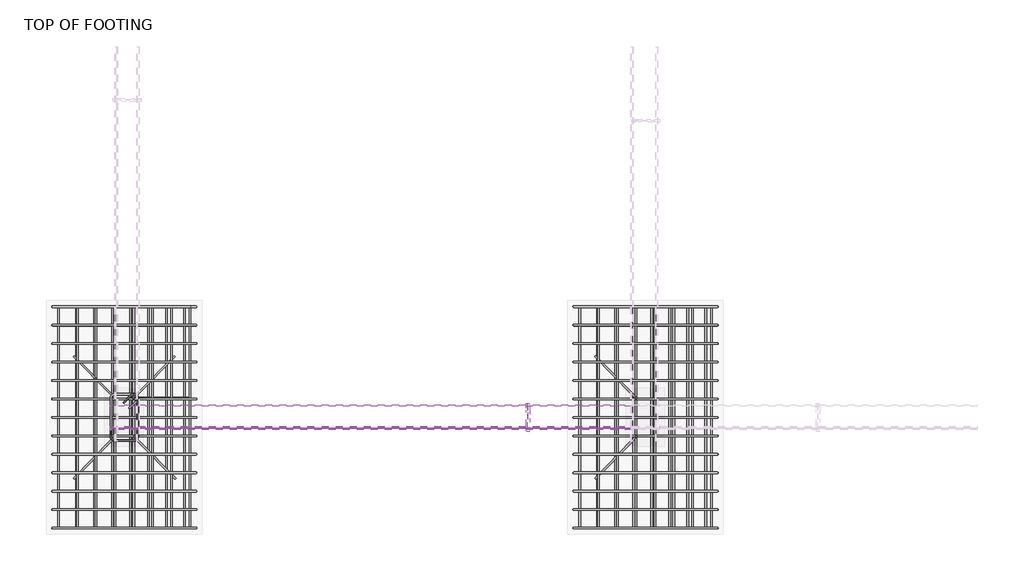
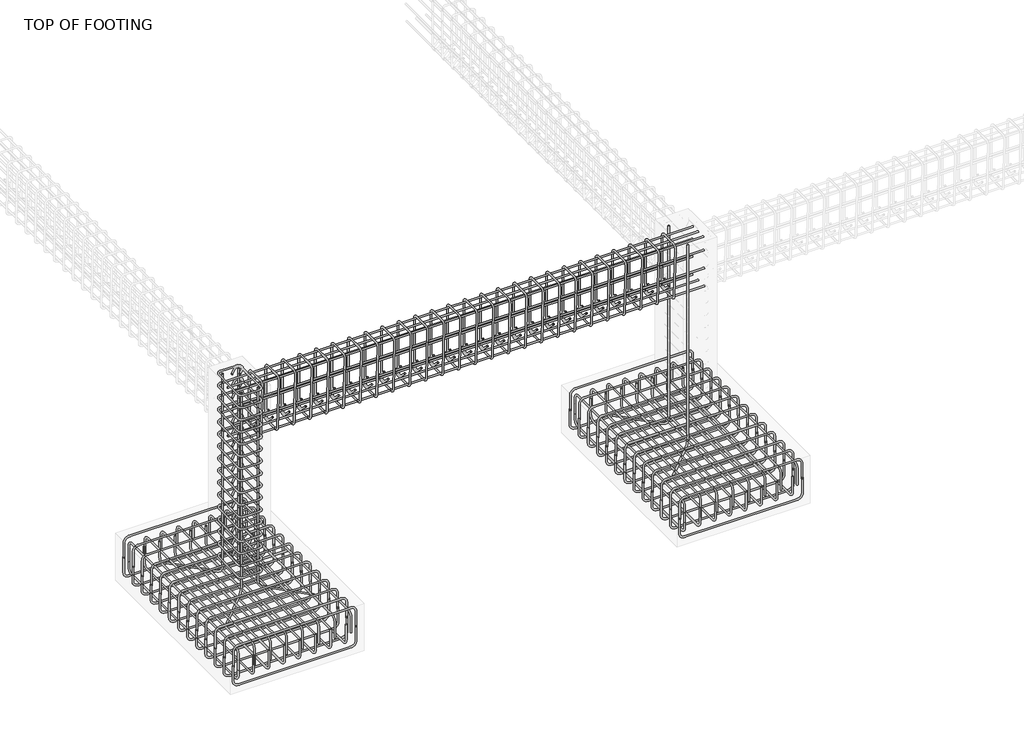
# One storey, part 2 of 21: 23 reinforcing bars.
"""IFC4 building model written with IfcOpenShell, lengths in millimetres."""

from ifc_helpers import new_model, si_unit, point, frame, origin, place, context, project, spatial, polyline, circle_curve, trimmed, segment, composite_curve, source, transform, mapped, element, save
from ifc_brep_helpers import swept_disk

model = new_model("IFC4")

# Units and contexts
model_context = context("Model", 3, world=origin())
ifc_project = project(units=[si_unit("LENGTHUNIT", "METRE", prefix="MILLI")], contexts=[model_context])

# Site, building, storey
site = spatial("IfcSite", under=ifc_project)
building = spatial("IfcBuilding", under=site)
storey = spatial("IfcBuildingStorey", under=building, Name="TOP OF FOOTING", Elevation=-1828.8)

# Reinforcing bars
placement = place(None, origin())
reinforcing_bar_shape = source(origin(), model_context, "Body", "SolidModel", [
    swept_disk(composite_curve([segment(polyline([(-13268.2584825, 443.1886958, -2045.4168622), (-13268.2584825, 443.1886958, -2192.7168622)]), True, "CONTINUOUS"), segment(trimmed(circle_curve(frame((-13314.6084825, 443.1886958, -2192.7168622), z_axis=(0.0, 1.0, 0.0), x_axis=(46.350000000000364, 0.0, 0.0)), 46.35), [point((-13268.2584825, 443.1886958, -2192.7168622))], [point((-13314.6084825, 443.1886958, -2239.0668622))], True, "CARTESIAN"), True, "CONTINUOUS"), segment(polyline([(-13314.6084825, 443.1886958, -2239.0668622), (-14329.2084825, 443.1886958, -2239.0668622)]), True, "CONTINUOUS"), segment(trimmed(circle_curve(frame((-14329.2084825, 443.1886958, -2192.7168622), z_axis=(0.0, 1.0, 0.0), x_axis=(0.0, 0.0, -46.34999999999991)), 46.35), [point((-14329.2084825, 443.1886958, -2239.0668622))], [point((-14375.5584825, 443.1886958, -2192.7168622))], True, "CARTESIAN"), True, "CONTINUOUS"), segment(polyline([(-14375.5584825, 443.1886958, -2192.7168622), (-14375.5584825, 443.1886958, -2045.4168622)]), True, "CONTINUOUS")], self_intersect=False), 6.35),
])
element("IfcReinforcingBar", 1, at=placement, inside=storey, context=model_context, shape_type="MappedRepresentation", body=[
    mapped(reinforcing_bar_shape, transform((0.0, 0.0, 0.0), x_axis=(1.0, 0.0, 0.0), y_axis=(0.0, 1.0, 0.0), z_axis=(0.0, 0.0, 1.0))),
    mapped(reinforcing_bar_shape, transform((0.0, -142.275, 0.0), x_axis=(1.0, 0.0, 0.0), y_axis=(0.0, 1.0, 0.0), z_axis=(0.0, 0.0, 1.0))),
    mapped(reinforcing_bar_shape, transform((0.0, -284.55, 0.0), x_axis=(1.0, 0.0, 0.0), y_axis=(0.0, 1.0, 0.0), z_axis=(0.0, 0.0, 1.0))),
    mapped(reinforcing_bar_shape, transform((0.0, -426.825, 0.0), x_axis=(1.0, 0.0, 0.0), y_axis=(0.0, 1.0, 0.0), z_axis=(0.0, 0.0, 1.0))),
    mapped(reinforcing_bar_shape, transform((0.0, -569.1, 0.0), x_axis=(1.0, 0.0, 0.0), y_axis=(0.0, 1.0, 0.0), z_axis=(0.0, 0.0, 1.0))),
    mapped(reinforcing_bar_shape, transform((0.0, -711.375, 0.0), x_axis=(1.0, 0.0, 0.0), y_axis=(0.0, 1.0, 0.0), z_axis=(0.0, 0.0, 1.0))),
    mapped(reinforcing_bar_shape, transform((0.0, -853.65, 0.0), x_axis=(1.0, 0.0, 0.0), y_axis=(0.0, 1.0, 0.0), z_axis=(0.0, 0.0, 1.0))),
    mapped(reinforcing_bar_shape, transform((0.0, -995.925, 0.0), x_axis=(1.0, 0.0, 0.0), y_axis=(0.0, 1.0, 0.0), z_axis=(0.0, 0.0, 1.0))),
    mapped(reinforcing_bar_shape, transform((0.0, -1138.2, 0.0), x_axis=(1.0, 0.0, 0.0), y_axis=(0.0, 1.0, 0.0), z_axis=(0.0, 0.0, 1.0))),
    mapped(reinforcing_bar_shape, transform((0.0, -1280.475, 0.0), x_axis=(1.0, 0.0, 0.0), y_axis=(0.0, 1.0, 0.0), z_axis=(0.0, 0.0, 1.0))),
    mapped(reinforcing_bar_shape, transform((0.0, -1422.75, 0.0), x_axis=(1.0, 0.0, 0.0), y_axis=(0.0, 1.0, 0.0), z_axis=(0.0, 0.0, 1.0))),
    mapped(reinforcing_bar_shape, transform((0.0, -1565.025, 0.0), x_axis=(1.0, 0.0, 0.0), y_axis=(0.0, 1.0, 0.0), z_axis=(0.0, 0.0, 1.0))),
    mapped(reinforcing_bar_shape, transform((0.0, -1707.3, 0.0), x_axis=(1.0, 0.0, 0.0), y_axis=(0.0, 1.0, 0.0), z_axis=(0.0, 0.0, 1.0))),
])
reinforcing_bar_2_shape = source(origin(), model_context, "Body", "SolidModel", [
    swept_disk(composite_curve([segment(polyline([(-14372.2274202, 443.1886958, -2057.1074344), (-14372.2274202, 443.1886958, -1909.8074344)]), True, "CONTINUOUS"), segment(trimmed(circle_curve(frame((-14325.8774202, 443.1886958, -1909.8074344), z_axis=(0.0, 1.0, 0.0), x_axis=(-46.350000000000364, 0.0, 0.0)), 46.35), [point((-14372.2274202, 443.1886958, -1909.8074344))], [point((-14325.8774202, 443.1886958, -1863.4574344))], True, "CARTESIAN"), True, "CONTINUOUS"), segment(polyline([(-14325.8774202, 443.1886958, -1863.4574344), (-13316.98705, 443.1886958, -1863.4574344)]), True, "CONTINUOUS"), segment(trimmed(circle_curve(frame((-13316.98705, 443.1886958, -1909.8074344), z_axis=(0.0, 1.0, 0.0), x_axis=(0.0, 0.0, 46.34999999999991)), 46.35), [point((-13316.98705, 443.1886958, -1863.4574344))], [point((-13270.63705, 443.1886958, -1909.8074344))], True, "CARTESIAN"), True, "CONTINUOUS"), segment(polyline([(-13270.63705, 443.1886958, -1909.8074344), (-13270.63705, 443.1886958, -2057.1074344)]), True, "CONTINUOUS")], self_intersect=False), 6.35),
])
element("IfcReinforcingBar", 2, at=placement, inside=storey, context=model_context, shape_type="MappedRepresentation", body=[
    mapped(reinforcing_bar_2_shape, transform((0.0, 0.0, 0.0), x_axis=(1.0, 0.0, 0.0), y_axis=(0.0, 1.0, 0.0), z_axis=(0.0, 0.0, 1.0))),
    mapped(reinforcing_bar_2_shape, transform((0.0, -142.275, 0.0), x_axis=(1.0, 0.0, 0.0), y_axis=(0.0, 1.0, 0.0), z_axis=(0.0, 0.0, 1.0))),
    mapped(reinforcing_bar_2_shape, transform((0.0, -284.55, 0.0), x_axis=(1.0, 0.0, 0.0), y_axis=(0.0, 1.0, 0.0), z_axis=(0.0, 0.0, 1.0))),
    mapped(reinforcing_bar_2_shape, transform((0.0, -426.825, 0.0), x_axis=(1.0, 0.0, 0.0), y_axis=(0.0, 1.0, 0.0), z_axis=(0.0, 0.0, 1.0))),
    mapped(reinforcing_bar_2_shape, transform((0.0, -569.1, 0.0), x_axis=(1.0, 0.0, 0.0), y_axis=(0.0, 1.0, 0.0), z_axis=(0.0, 0.0, 1.0))),
    mapped(reinforcing_bar_2_shape, transform((0.0, -711.375, 0.0), x_axis=(1.0, 0.0, 0.0), y_axis=(0.0, 1.0, 0.0), z_axis=(0.0, 0.0, 1.0))),
    mapped(reinforcing_bar_2_shape, transform((0.0, -853.65, 0.0), x_axis=(1.0, 0.0, 0.0), y_axis=(0.0, 1.0, 0.0), z_axis=(0.0, 0.0, 1.0))),
    mapped(reinforcing_bar_2_shape, transform((0.0, -995.925, 0.0), x_axis=(1.0, 0.0, 0.0), y_axis=(0.0, 1.0, 0.0), z_axis=(0.0, 0.0, 1.0))),
    mapped(reinforcing_bar_2_shape, transform((0.0, -1138.2, 0.0), x_axis=(1.0, 0.0, 0.0), y_axis=(0.0, 1.0, 0.0), z_axis=(0.0, 0.0, 1.0))),
    mapped(reinforcing_bar_2_shape, transform((0.0, -1280.475, 0.0), x_axis=(1.0, 0.0, 0.0), y_axis=(0.0, 1.0, 0.0), z_axis=(0.0, 0.0, 1.0))),
    mapped(reinforcing_bar_2_shape, transform((0.0, -1422.75, 0.0), x_axis=(1.0, 0.0, 0.0), y_axis=(0.0, 1.0, 0.0), z_axis=(0.0, 0.0, 1.0))),
    mapped(reinforcing_bar_2_shape, transform((0.0, -1565.025, 0.0), x_axis=(1.0, 0.0, 0.0), y_axis=(0.0, 1.0, 0.0), z_axis=(0.0, 0.0, 1.0))),
    mapped(reinforcing_bar_2_shape, transform((0.0, -1707.3, 0.0), x_axis=(1.0, 0.0, 0.0), y_axis=(0.0, 1.0, 0.0), z_axis=(0.0, 0.0, 1.0))),
])
reinforcing_bar_3_shape = source(origin(), model_context, "Body", "SolidModel", [
    swept_disk(composite_curve([segment(polyline([(-13314.2120502, 443.1886958, -2099.3509187), (-13314.2120502, 443.1886958, -1952.0509187)]), True, "CONTINUOUS"), segment(trimmed(circle_curve(frame((-13314.2120502, 396.8386958, -1952.0509187), z_axis=(1.0, 0.0, 0.0), x_axis=(0.0, 46.35000000000002, 0.0)), 46.35), [point((-13314.2120502, 443.1886958, -1952.0509187))], [point((-13314.2120502, 396.8386958, -1905.7009187))], True, "CARTESIAN"), True, "CONTINUOUS"), segment(polyline([(-13314.2120502, 396.8386958, -1905.7009187), (-13314.2120502, -1217.7613042, -1905.7009187)]), True, "CONTINUOUS"), segment(trimmed(circle_curve(frame((-13314.2120502, -1217.7613042, -1952.0509187), z_axis=(1.0, 0.0, 0.0), x_axis=(0.0, 0.0, 46.34999999999991)), 46.35), [point((-13314.2120502, -1217.7613042, -1905.7009187))], [point((-13314.2120502, -1264.1113042, -1952.0509187))], True, "CARTESIAN"), True, "CONTINUOUS"), segment(polyline([(-13314.2120502, -1264.1113042, -1952.0509187), (-13314.2120502, -1264.1113042, -2099.3509187)]), True, "CONTINUOUS")], self_intersect=False), 6.35),
])
element("IfcReinforcingBar", 3, at=placement, inside=storey, context=model_context, shape_type="MappedRepresentation", body=[
    mapped(reinforcing_bar_3_shape, transform((0.0, 0.0, 0.0), x_axis=(1.0, 0.0, 0.0), y_axis=(0.0, 1.0, 0.0), z_axis=(0.0, 0.0, 1.0))),
    mapped(reinforcing_bar_3_shape, transform((-145.0295561, 0.0, 0.0), x_axis=(1.0, 0.0, 0.0), y_axis=(0.0, 1.0, 0.0), z_axis=(0.0, 0.0, 1.0))),
    mapped(reinforcing_bar_3_shape, transform((-290.0591123, 0.0, 0.0), x_axis=(1.0, 0.0, 0.0), y_axis=(0.0, 1.0, 0.0), z_axis=(0.0, 0.0, 1.0))),
    mapped(reinforcing_bar_3_shape, transform((-435.0886684, 0.0, 0.0), x_axis=(1.0, 0.0, 0.0), y_axis=(0.0, 1.0, 0.0), z_axis=(0.0, 0.0, 1.0))),
    mapped(reinforcing_bar_3_shape, transform((-580.1182245, 0.0, 0.0), x_axis=(1.0, 0.0, 0.0), y_axis=(0.0, 1.0, 0.0), z_axis=(0.0, 0.0, 1.0))),
    mapped(reinforcing_bar_3_shape, transform((-725.1477807, 0.0, 0.0), x_axis=(1.0, 0.0, 0.0), y_axis=(0.0, 1.0, 0.0), z_axis=(0.0, 0.0, 1.0))),
    mapped(reinforcing_bar_3_shape, transform((-870.1773368, 0.0, 0.0), x_axis=(1.0, 0.0, 0.0), y_axis=(0.0, 1.0, 0.0), z_axis=(0.0, 0.0, 1.0))),
    mapped(reinforcing_bar_3_shape, transform((-1015.206893, 0.0, 0.0), x_axis=(1.0, 0.0, 0.0), y_axis=(0.0, 1.0, 0.0), z_axis=(0.0, 0.0, 1.0))),
])
reinforcing_bar_4_shape = source(origin(), model_context, "Body", "SolidModel", [
    swept_disk(composite_curve([segment(polyline([(-14329.4189432, 443.1886958, -2006.0306816), (-14329.4189432, 443.1886958, -2153.3306816)]), True, "CONTINUOUS"), segment(trimmed(circle_curve(frame((-14329.4189432, 396.8386958, -2153.3306816), z_axis=(-1.0, 0.0, 0.0), x_axis=(0.0, 46.35000000000002, 0.0)), 46.35), [point((-14329.4189432, 443.1886958, -2153.3306816))], [point((-14329.4189432, 396.8386958, -2199.6806816))], True, "CARTESIAN"), True, "CONTINUOUS"), segment(polyline([(-14329.4189432, 396.8386958, -2199.6806816), (-14329.4189432, -1217.7613042, -2199.6806816)]), True, "CONTINUOUS"), segment(trimmed(circle_curve(frame((-14329.4189432, -1217.7613042, -2153.3306816), z_axis=(-1.0, 0.0, 0.0), x_axis=(0.0, 0.0, -46.34999999999991)), 46.35), [point((-14329.4189432, -1217.7613042, -2199.6806816))], [point((-14329.4189432, -1264.1113042, -2153.3306816))], True, "CARTESIAN"), True, "CONTINUOUS"), segment(polyline([(-14329.4189432, -1264.1113042, -2153.3306816), (-14329.4189432, -1264.1113042, -2006.0306816)]), True, "CONTINUOUS")], self_intersect=False), 6.35),
])
element("IfcReinforcingBar", 4, at=placement, inside=storey, context=model_context, shape_type="MappedRepresentation", body=[
    mapped(reinforcing_bar_4_shape, transform((0.0, 0.0, 0.0), x_axis=(1.0, 0.0, 0.0), y_axis=(0.0, 1.0, 0.0), z_axis=(0.0, 0.0, 1.0))),
    mapped(reinforcing_bar_4_shape, transform((138.8823255, 0.0, 0.0), x_axis=(1.0, 0.0, 0.0), y_axis=(0.0, 1.0, 0.0), z_axis=(0.0, 0.0, 1.0))),
    mapped(reinforcing_bar_4_shape, transform((277.7646509, 0.0, 0.0), x_axis=(1.0, 0.0, 0.0), y_axis=(0.0, 1.0, 0.0), z_axis=(0.0, 0.0, 1.0))),
    mapped(reinforcing_bar_4_shape, transform((416.6469764, 0.0, 0.0), x_axis=(1.0, 0.0, 0.0), y_axis=(0.0, 1.0, 0.0), z_axis=(0.0, 0.0, 1.0))),
    mapped(reinforcing_bar_4_shape, transform((555.5293018, 0.0, 0.0), x_axis=(1.0, 0.0, 0.0), y_axis=(0.0, 1.0, 0.0), z_axis=(0.0, 0.0, 1.0))),
    mapped(reinforcing_bar_4_shape, transform((694.4116273, 0.0, 0.0), x_axis=(1.0, 0.0, 0.0), y_axis=(0.0, 1.0, 0.0), z_axis=(0.0, 0.0, 1.0))),
    mapped(reinforcing_bar_4_shape, transform((833.2939527, 0.0, 0.0), x_axis=(1.0, 0.0, 0.0), y_axis=(0.0, 1.0, 0.0), z_axis=(0.0, 0.0, 1.0))),
    mapped(reinforcing_bar_4_shape, transform((972.1762782, 0.0, 0.0), x_axis=(1.0, 0.0, 0.0), y_axis=(0.0, 1.0, 0.0), z_axis=(0.0, 0.0, 1.0))),
])
reinforcing_bar_5_shape = source(origin(), model_context, "Body", "SolidModel", [
    swept_disk(composite_curve([segment(polyline([(-9248.5313539, 443.1886958, -2045.4168622), (-9248.5313539, 443.1886958, -2192.7168622)]), True, "CONTINUOUS"), segment(trimmed(circle_curve(frame((-9294.8813539, 443.1886958, -2192.7168622), z_axis=(0.0, 1.0, 0.0), x_axis=(46.350000000000364, 0.0, 0.0)), 46.35), [point((-9248.5313539, 443.1886958, -2192.7168622))], [point((-9294.8813539, 443.1886958, -2239.0668622))], True, "CARTESIAN"), True, "CONTINUOUS"), segment(polyline([(-9294.8813539, 443.1886958, -2239.0668622), (-10309.4813539, 443.1886958, -2239.0668622)]), True, "CONTINUOUS"), segment(trimmed(circle_curve(frame((-10309.4813539, 443.1886958, -2192.7168622), z_axis=(0.0, 1.0, 0.0), x_axis=(0.0, 0.0, -46.34999999999991)), 46.35), [point((-10309.4813539, 443.1886958, -2239.0668622))], [point((-10355.8313539, 443.1886958, -2192.7168622))], True, "CARTESIAN"), True, "CONTINUOUS"), segment(polyline([(-10355.8313539, 443.1886958, -2192.7168622), (-10355.8313539, 443.1886958, -2045.4168622)]), True, "CONTINUOUS")], self_intersect=False), 6.35),
])
element("IfcReinforcingBar", 5, at=placement, inside=storey, context=model_context, shape_type="MappedRepresentation", body=[
    mapped(reinforcing_bar_5_shape, transform((0.0, 0.0, 0.0), x_axis=(1.0, 0.0, 0.0), y_axis=(0.0, 1.0, 0.0), z_axis=(0.0, 0.0, 1.0))),
    mapped(reinforcing_bar_5_shape, transform((0.0, -142.275, 0.0), x_axis=(1.0, 0.0, 0.0), y_axis=(0.0, 1.0, 0.0), z_axis=(0.0, 0.0, 1.0))),
    mapped(reinforcing_bar_5_shape, transform((0.0, -284.55, 0.0), x_axis=(1.0, 0.0, 0.0), y_axis=(0.0, 1.0, 0.0), z_axis=(0.0, 0.0, 1.0))),
    mapped(reinforcing_bar_5_shape, transform((0.0, -426.825, 0.0), x_axis=(1.0, 0.0, 0.0), y_axis=(0.0, 1.0, 0.0), z_axis=(0.0, 0.0, 1.0))),
    mapped(reinforcing_bar_5_shape, transform((0.0, -569.1, 0.0), x_axis=(1.0, 0.0, 0.0), y_axis=(0.0, 1.0, 0.0), z_axis=(0.0, 0.0, 1.0))),
    mapped(reinforcing_bar_5_shape, transform((0.0, -711.375, 0.0), x_axis=(1.0, 0.0, 0.0), y_axis=(0.0, 1.0, 0.0), z_axis=(0.0, 0.0, 1.0))),
    mapped(reinforcing_bar_5_shape, transform((0.0, -853.65, 0.0), x_axis=(1.0, 0.0, 0.0), y_axis=(0.0, 1.0, 0.0), z_axis=(0.0, 0.0, 1.0))),
    mapped(reinforcing_bar_5_shape, transform((0.0, -995.925, 0.0), x_axis=(1.0, 0.0, 0.0), y_axis=(0.0, 1.0, 0.0), z_axis=(0.0, 0.0, 1.0))),
    mapped(reinforcing_bar_5_shape, transform((0.0, -1138.2, 0.0), x_axis=(1.0, 0.0, 0.0), y_axis=(0.0, 1.0, 0.0), z_axis=(0.0, 0.0, 1.0))),
    mapped(reinforcing_bar_5_shape, transform((0.0, -1280.475, 0.0), x_axis=(1.0, 0.0, 0.0), y_axis=(0.0, 1.0, 0.0), z_axis=(0.0, 0.0, 1.0))),
    mapped(reinforcing_bar_5_shape, transform((0.0, -1422.75, 0.0), x_axis=(1.0, 0.0, 0.0), y_axis=(0.0, 1.0, 0.0), z_axis=(0.0, 0.0, 1.0))),
    mapped(reinforcing_bar_5_shape, transform((0.0, -1565.025, 0.0), x_axis=(1.0, 0.0, 0.0), y_axis=(0.0, 1.0, 0.0), z_axis=(0.0, 0.0, 1.0))),
    mapped(reinforcing_bar_5_shape, transform((0.0, -1707.3, 0.0), x_axis=(1.0, 0.0, 0.0), y_axis=(0.0, 1.0, 0.0), z_axis=(0.0, 0.0, 1.0))),
])
reinforcing_bar_6_shape = source(origin(), model_context, "Body", "SolidModel", [
    swept_disk(composite_curve([segment(polyline([(-10352.5002917, 443.1886958, -2057.1074344), (-10352.5002917, 443.1886958, -1909.8074344)]), True, "CONTINUOUS"), segment(trimmed(circle_curve(frame((-10306.1502917, 443.1886958, -1909.8074344), z_axis=(0.0, 1.0, 0.0), x_axis=(-46.350000000000364, 0.0, 0.0)), 46.35), [point((-10352.5002917, 443.1886958, -1909.8074344))], [point((-10306.1502917, 443.1886958, -1863.4574344))], True, "CARTESIAN"), True, "CONTINUOUS"), segment(polyline([(-10306.1502917, 443.1886958, -1863.4574344), (-9297.2599214, 443.1886958, -1863.4574344)]), True, "CONTINUOUS"), segment(trimmed(circle_curve(frame((-9297.2599214, 443.1886958, -1909.8074344), z_axis=(0.0, 1.0, 0.0), x_axis=(0.0, 0.0, 46.34999999999991)), 46.35), [point((-9297.2599214, 443.1886958, -1863.4574344))], [point((-9250.9099214, 443.1886958, -1909.8074344))], True, "CARTESIAN"), True, "CONTINUOUS"), segment(polyline([(-9250.9099214, 443.1886958, -1909.8074344), (-9250.9099214, 443.1886958, -2057.1074344)]), True, "CONTINUOUS")], self_intersect=False), 6.35),
])
element("IfcReinforcingBar", 6, at=placement, inside=storey, context=model_context, shape_type="MappedRepresentation", body=[
    mapped(reinforcing_bar_6_shape, transform((0.0, 0.0, 0.0), x_axis=(1.0, 0.0, 0.0), y_axis=(0.0, 1.0, 0.0), z_axis=(0.0, 0.0, 1.0))),
    mapped(reinforcing_bar_6_shape, transform((0.0, -142.275, 0.0), x_axis=(1.0, 0.0, 0.0), y_axis=(0.0, 1.0, 0.0), z_axis=(0.0, 0.0, 1.0))),
    mapped(reinforcing_bar_6_shape, transform((0.0, -284.55, 0.0), x_axis=(1.0, 0.0, 0.0), y_axis=(0.0, 1.0, 0.0), z_axis=(0.0, 0.0, 1.0))),
    mapped(reinforcing_bar_6_shape, transform((0.0, -426.825, 0.0), x_axis=(1.0, 0.0, 0.0), y_axis=(0.0, 1.0, 0.0), z_axis=(0.0, 0.0, 1.0))),
    mapped(reinforcing_bar_6_shape, transform((0.0, -569.1, 0.0), x_axis=(1.0, 0.0, 0.0), y_axis=(0.0, 1.0, 0.0), z_axis=(0.0, 0.0, 1.0))),
    mapped(reinforcing_bar_6_shape, transform((0.0, -711.375, 0.0), x_axis=(1.0, 0.0, 0.0), y_axis=(0.0, 1.0, 0.0), z_axis=(0.0, 0.0, 1.0))),
    mapped(reinforcing_bar_6_shape, transform((0.0, -853.65, 0.0), x_axis=(1.0, 0.0, 0.0), y_axis=(0.0, 1.0, 0.0), z_axis=(0.0, 0.0, 1.0))),
    mapped(reinforcing_bar_6_shape, transform((0.0, -995.925, 0.0), x_axis=(1.0, 0.0, 0.0), y_axis=(0.0, 1.0, 0.0), z_axis=(0.0, 0.0, 1.0))),
    mapped(reinforcing_bar_6_shape, transform((0.0, -1138.2, 0.0), x_axis=(1.0, 0.0, 0.0), y_axis=(0.0, 1.0, 0.0), z_axis=(0.0, 0.0, 1.0))),
    mapped(reinforcing_bar_6_shape, transform((0.0, -1280.475, 0.0), x_axis=(1.0, 0.0, 0.0), y_axis=(0.0, 1.0, 0.0), z_axis=(0.0, 0.0, 1.0))),
    mapped(reinforcing_bar_6_shape, transform((0.0, -1422.75, 0.0), x_axis=(1.0, 0.0, 0.0), y_axis=(0.0, 1.0, 0.0), z_axis=(0.0, 0.0, 1.0))),
    mapped(reinforcing_bar_6_shape, transform((0.0, -1565.025, 0.0), x_axis=(1.0, 0.0, 0.0), y_axis=(0.0, 1.0, 0.0), z_axis=(0.0, 0.0, 1.0))),
    mapped(reinforcing_bar_6_shape, transform((0.0, -1707.3, 0.0), x_axis=(1.0, 0.0, 0.0), y_axis=(0.0, 1.0, 0.0), z_axis=(0.0, 0.0, 1.0))),
])
reinforcing_bar_7_shape = source(origin(), model_context, "Body", "SolidModel", [
    swept_disk(composite_curve([segment(polyline([(-9294.4849216, 443.1886958, -2099.3509187), (-9294.4849216, 443.1886958, -1952.0509187)]), True, "CONTINUOUS"), segment(trimmed(circle_curve(frame((-9294.4849216, 396.8386958, -1952.0509187), z_axis=(1.0, 0.0, 0.0), x_axis=(0.0, 46.35000000000002, 0.0)), 46.35), [point((-9294.4849216, 443.1886958, -1952.0509187))], [point((-9294.4849216, 396.8386958, -1905.7009187))], True, "CARTESIAN"), True, "CONTINUOUS"), segment(polyline([(-9294.4849216, 396.8386958, -1905.7009187), (-9294.4849216, -1217.7613042, -1905.7009187)]), True, "CONTINUOUS"), segment(trimmed(circle_curve(frame((-9294.4849216, -1217.7613042, -1952.0509187), z_axis=(1.0, 0.0, 0.0), x_axis=(0.0, 0.0, 46.34999999999991)), 46.35), [point((-9294.4849216, -1217.7613042, -1905.7009187))], [point((-9294.4849216, -1264.1113042, -1952.0509187))], True, "CARTESIAN"), True, "CONTINUOUS"), segment(polyline([(-9294.4849216, -1264.1113042, -1952.0509187), (-9294.4849216, -1264.1113042, -2099.3509187)]), True, "CONTINUOUS")], self_intersect=False), 6.35),
])
element("IfcReinforcingBar", 7, at=placement, inside=storey, context=model_context, shape_type="MappedRepresentation", body=[
    mapped(reinforcing_bar_7_shape, transform((0.0, 0.0, 0.0), x_axis=(1.0, 0.0, 0.0), y_axis=(0.0, 1.0, 0.0), z_axis=(0.0, 0.0, 1.0))),
    mapped(reinforcing_bar_7_shape, transform((-145.0295561, 0.0, 0.0), x_axis=(1.0, 0.0, 0.0), y_axis=(0.0, 1.0, 0.0), z_axis=(0.0, 0.0, 1.0))),
    mapped(reinforcing_bar_7_shape, transform((-290.0591123, 0.0, 0.0), x_axis=(1.0, 0.0, 0.0), y_axis=(0.0, 1.0, 0.0), z_axis=(0.0, 0.0, 1.0))),
    mapped(reinforcing_bar_7_shape, transform((-435.0886684, 0.0, 0.0), x_axis=(1.0, 0.0, 0.0), y_axis=(0.0, 1.0, 0.0), z_axis=(0.0, 0.0, 1.0))),
    mapped(reinforcing_bar_7_shape, transform((-580.1182245, 0.0, 0.0), x_axis=(1.0, 0.0, 0.0), y_axis=(0.0, 1.0, 0.0), z_axis=(0.0, 0.0, 1.0))),
    mapped(reinforcing_bar_7_shape, transform((-725.1477807, 0.0, 0.0), x_axis=(1.0, 0.0, 0.0), y_axis=(0.0, 1.0, 0.0), z_axis=(0.0, 0.0, 1.0))),
    mapped(reinforcing_bar_7_shape, transform((-870.1773368, 0.0, 0.0), x_axis=(1.0, 0.0, 0.0), y_axis=(0.0, 1.0, 0.0), z_axis=(0.0, 0.0, 1.0))),
    mapped(reinforcing_bar_7_shape, transform((-1015.206893, 0.0, 0.0), x_axis=(1.0, 0.0, 0.0), y_axis=(0.0, 1.0, 0.0), z_axis=(0.0, 0.0, 1.0))),
])
reinforcing_bar_8_shape = source(origin(), model_context, "Body", "SolidModel", [
    swept_disk(composite_curve([segment(polyline([(-10309.6918146, 443.1886958, -2006.0306816), (-10309.6918146, 443.1886958, -2153.3306816)]), True, "CONTINUOUS"), segment(trimmed(circle_curve(frame((-10309.6918146, 396.8386958, -2153.3306816), z_axis=(-1.0, 0.0, 0.0), x_axis=(0.0, 46.35000000000002, 0.0)), 46.35), [point((-10309.6918146, 443.1886958, -2153.3306816))], [point((-10309.6918146, 396.8386958, -2199.6806816))], True, "CARTESIAN"), True, "CONTINUOUS"), segment(polyline([(-10309.6918146, 396.8386958, -2199.6806816), (-10309.6918146, -1217.7613042, -2199.6806816)]), True, "CONTINUOUS"), segment(trimmed(circle_curve(frame((-10309.6918146, -1217.7613042, -2153.3306816), z_axis=(-1.0, 0.0, 0.0), x_axis=(0.0, 0.0, -46.34999999999991)), 46.35), [point((-10309.6918146, -1217.7613042, -2199.6806816))], [point((-10309.6918146, -1264.1113042, -2153.3306816))], True, "CARTESIAN"), True, "CONTINUOUS"), segment(polyline([(-10309.6918146, -1264.1113042, -2153.3306816), (-10309.6918146, -1264.1113042, -2006.0306816)]), True, "CONTINUOUS")], self_intersect=False), 6.35),
])
element("IfcReinforcingBar", 8, at=placement, inside=storey, context=model_context, shape_type="MappedRepresentation", body=[
    mapped(reinforcing_bar_8_shape, transform((0.0, 0.0, 0.0), x_axis=(1.0, 0.0, 0.0), y_axis=(0.0, 1.0, 0.0), z_axis=(0.0, 0.0, 1.0))),
    mapped(reinforcing_bar_8_shape, transform((138.8823255, 0.0, 0.0), x_axis=(1.0, 0.0, 0.0), y_axis=(0.0, 1.0, 0.0), z_axis=(0.0, 0.0, 1.0))),
    mapped(reinforcing_bar_8_shape, transform((277.7646509, 0.0, 0.0), x_axis=(1.0, 0.0, 0.0), y_axis=(0.0, 1.0, 0.0), z_axis=(0.0, 0.0, 1.0))),
    mapped(reinforcing_bar_8_shape, transform((416.6469764, 0.0, 0.0), x_axis=(1.0, 0.0, 0.0), y_axis=(0.0, 1.0, 0.0), z_axis=(0.0, 0.0, 1.0))),
    mapped(reinforcing_bar_8_shape, transform((555.5293018, 0.0, 0.0), x_axis=(1.0, 0.0, 0.0), y_axis=(0.0, 1.0, 0.0), z_axis=(0.0, 0.0, 1.0))),
    mapped(reinforcing_bar_8_shape, transform((694.4116273, 0.0, 0.0), x_axis=(1.0, 0.0, 0.0), y_axis=(0.0, 1.0, 0.0), z_axis=(0.0, 0.0, 1.0))),
    mapped(reinforcing_bar_8_shape, transform((833.2939527, 0.0, 0.0), x_axis=(1.0, 0.0, 0.0), y_axis=(0.0, 1.0, 0.0), z_axis=(0.0, 0.0, 1.0))),
    mapped(reinforcing_bar_8_shape, transform((972.1762782, 0.0, 0.0), x_axis=(1.0, 0.0, 0.0), y_axis=(0.0, 1.0, 0.0), z_axis=(0.0, 0.0, 1.0))),
])
reinforcing_bar_9_shape = source(origin(), model_context, "Body", "SolidModel", [
    swept_disk(composite_curve([segment(polyline([(-13827.5198431, -296.7370695, -46.35), (-13771.7762801, -240.9935066, -46.35)]), True, "CONTINUOUS"), segment(trimmed(circle_curve(frame((-13749.6084825, -263.1613042, -46.35), z_axis=(0.0, 0.0, -1.0), x_axis=(-22.167797600000995, 22.16779760000003, 0.0)), 31.35), [point((-13771.7762801, -240.9935066, -46.35))], [point((-13718.2584825, -263.1613042, -46.35))], True, "CARTESIAN"), True, "CONTINUOUS"), segment(polyline([(-13718.2584825, -263.1613042, -46.35), (-13718.2584825, -557.7613042, -46.35)]), True, "CONTINUOUS"), segment(trimmed(circle_curve(frame((-13749.6084825, -557.7613042, -46.35), z_axis=(0.0, 0.0, -1.0), x_axis=(31.350000000000364, 0.0, 0.0)), 31.35), [point((-13718.2584825, -557.7613042, -46.35))], [point((-13749.6084825, -589.1113042, -46.35))], True, "CARTESIAN"), True, "CONTINUOUS"), segment(polyline([(-13749.6084825, -589.1113042, -46.35), (-13894.2084825, -589.1113042, -46.35)]), True, "CONTINUOUS"), segment(trimmed(circle_curve(frame((-13894.2084825, -557.7810893, -45.2363875), z_axis=(0.0, 0.035521928334481916, -0.9993688971583016), x_axis=(0.0, -31.330214899999987, -1.1136125000000021)), 31.35), [point((-13894.2084825, -589.1113042, -46.35))], [point((-13925.5584825, -557.7810893, -45.2363875))], True, "CARTESIAN"), True, "CONTINUOUS"), segment(polyline([(-13925.5584825, -557.7810893, -45.2363875), (-13925.5584825, -263.1415191, -34.7636125)]), True, "CONTINUOUS"), segment(trimmed(circle_curve(frame((-13894.2084825, -263.1415191, -34.7636125), z_axis=(0.0, 0.035521928334481916, -0.9993688971583016), x_axis=(-31.350000000000364, 0.0, 0.0)), 31.35), [point((-13925.5584825, -263.1415191, -34.7636125))], [point((-13894.2084825, -231.8113042, -33.65))], True, "CARTESIAN"), True, "CONTINUOUS"), segment(polyline([(-13894.2084825, -231.8113042, -33.65), (-13749.6084825, -231.8113042, -33.65)]), True, "CONTINUOUS"), segment(trimmed(circle_curve(frame((-13749.6084825, -263.1613042, -33.65), z_axis=(0.0, 0.0, -1.0), x_axis=(0.0, 31.350000000000023, 0.0)), 31.35), [point((-13749.6084825, -231.8113042, -33.65))], [point((-13727.4406849, -285.3291018, -33.65))], True, "CARTESIAN"), True, "CONTINUOUS"), segment(polyline([(-13727.4406849, -285.3291018, -33.65), (-13783.1842479, -341.0726647, -33.65)]), True, "CONTINUOUS")], self_intersect=False), 6.35),
])
element("IfcReinforcingBar", 9, at=placement, inside=storey, context=model_context, shape_type="MappedRepresentation", body=[
    mapped(reinforcing_bar_9_shape, transform((0.0, 0.0, 0.0), x_axis=(1.0, 0.0, 0.0), y_axis=(0.0, 1.0, 0.0), z_axis=(0.0, 0.0, 1.0))),
    mapped(reinforcing_bar_9_shape, transform((0.0, 0.0, -115.74), x_axis=(1.0, 0.0, 0.0), y_axis=(0.0, 1.0, 0.0), z_axis=(0.0, 0.0, 1.0))),
    mapped(reinforcing_bar_9_shape, transform((0.0, 0.0, -231.48), x_axis=(1.0, 0.0, 0.0), y_axis=(0.0, 1.0, 0.0), z_axis=(0.0, 0.0, 1.0))),
    mapped(reinforcing_bar_9_shape, transform((0.0, 0.0, -347.22), x_axis=(1.0, 0.0, 0.0), y_axis=(0.0, 1.0, 0.0), z_axis=(0.0, 0.0, 1.0))),
    mapped(reinforcing_bar_9_shape, transform((0.0, 0.0, -462.96), x_axis=(1.0, 0.0, 0.0), y_axis=(0.0, 1.0, 0.0), z_axis=(0.0, 0.0, 1.0))),
    mapped(reinforcing_bar_9_shape, transform((0.0, 0.0, -578.7), x_axis=(1.0, 0.0, 0.0), y_axis=(0.0, 1.0, 0.0), z_axis=(0.0, 0.0, 1.0))),
    mapped(reinforcing_bar_9_shape, transform((0.0, 0.0, -694.44), x_axis=(1.0, 0.0, 0.0), y_axis=(0.0, 1.0, 0.0), z_axis=(0.0, 0.0, 1.0))),
    mapped(reinforcing_bar_9_shape, transform((0.0, 0.0, -810.18), x_axis=(1.0, 0.0, 0.0), y_axis=(0.0, 1.0, 0.0), z_axis=(0.0, 0.0, 1.0))),
    mapped(reinforcing_bar_9_shape, transform((0.0, 0.0, -925.92), x_axis=(1.0, 0.0, 0.0), y_axis=(0.0, 1.0, 0.0), z_axis=(0.0, 0.0, 1.0))),
    mapped(reinforcing_bar_9_shape, transform((0.0, 0.0, -1041.66), x_axis=(1.0, 0.0, 0.0), y_axis=(0.0, 1.0, 0.0), z_axis=(0.0, 0.0, 1.0))),
    mapped(reinforcing_bar_9_shape, transform((0.0, 0.0, -1157.4), x_axis=(1.0, 0.0, 0.0), y_axis=(0.0, 1.0, 0.0), z_axis=(0.0, 0.0, 1.0))),
    mapped(reinforcing_bar_9_shape, transform((0.0, 0.0, -1273.14), x_axis=(1.0, 0.0, 0.0), y_axis=(0.0, 1.0, 0.0), z_axis=(0.0, 0.0, 1.0))),
    mapped(reinforcing_bar_9_shape, transform((0.0, 0.0, -1388.88), x_axis=(1.0, 0.0, 0.0), y_axis=(0.0, 1.0, 0.0), z_axis=(0.0, 0.0, 1.0))),
    mapped(reinforcing_bar_9_shape, transform((0.0, 0.0, -1504.62), x_axis=(1.0, 0.0, 0.0), y_axis=(0.0, 1.0, 0.0), z_axis=(0.0, 0.0, 1.0))),
    mapped(reinforcing_bar_9_shape, transform((0.0, 0.0, -1620.36), x_axis=(1.0, 0.0, 0.0), y_axis=(0.0, 1.0, 0.0), z_axis=(0.0, 0.0, 1.0))),
    mapped(reinforcing_bar_9_shape, transform((0.0, 0.0, -1736.1), x_axis=(1.0, 0.0, 0.0), y_axis=(0.0, 1.0, 0.0), z_axis=(0.0, 0.0, 1.0))),
])
element("IfcReinforcingBar", 10, at=placement, inside=storey, context=model_context, shape_type="SolidModel", body=[
    swept_disk(composite_curve([segment(polyline([(-13750.0878823, -262.059512, -40.0), (-13750.0878823, -262.059512, -1882.5259187)]), True, "CONTINUOUS"), segment(trimmed(circle_curve(frame((-13703.7378823, -262.059512, -1882.5259187), z_axis=(0.0, -1.0, 0.0), x_axis=(-46.350000000000364, 0.0, 0.0)), 46.35), [point((-13750.0878823, -262.059512, -1882.5259187))], [point((-13703.7378823, -262.059512, -1928.8759187))], True, "CARTESIAN"), True, "CONTINUOUS"), segment(polyline([(-13703.7378823, -262.059512, -1928.8759187), (-13314.2120502, -262.059512, -1928.8759187)]), True, "CONTINUOUS")], self_intersect=False), 6.35),
])
element("IfcReinforcingBar", 11, at=placement, inside=storey, context=model_context, shape_type="SolidModel", body=[
    swept_disk(composite_curve([segment(polyline([(-13750.0878823, -262.059512, -40.0), (-13750.0878823, -262.059512, -1882.5259187)]), True, "CONTINUOUS"), segment(trimmed(circle_curve(frame((-13717.6297647, -228.9718542, -1882.5259187), z_axis=(0.7138653253877265, -0.7002830122236834, 0.0), x_axis=(-32.45811760000106, -33.08765779999999, 0.0)), 46.35), [point((-13750.0878823, -262.059512, -1882.5259187))], [point((-13717.6297647, -228.9718542, -1928.8759187))], True, "CARTESIAN"), True, "CONTINUOUS"), segment(polyline([(-13717.6297647, -228.9718542, -1928.8759187), (-13432.8602442, 61.320903, -1928.8759187)]), True, "CONTINUOUS")], self_intersect=False), 6.35),
])
element("IfcReinforcingBar", 12, at=placement, inside=storey, context=model_context, shape_type="SolidModel", body=[
    swept_disk(composite_curve([segment(polyline([(-13893.7290828, -262.059512, -40.0), (-13893.7290828, -262.059512, -1882.5259187)]), True, "CONTINUOUS"), segment(trimmed(circle_curve(frame((-13926.1872004, -228.9718542, -1882.5259187), z_axis=(0.7138653253877092, 0.700283012223701, 0.0), x_axis=(32.45811759999924, -33.08765779999999, 0.0)), 46.35), [point((-13893.7290828, -262.059512, -1882.5259187))], [point((-13926.1872004, -228.9718542, -1928.8759187))], True, "CARTESIAN"), True, "CONTINUOUS"), segment(polyline([(-13926.1872004, -228.9718542, -1928.8759187), (-14210.9567208, 61.320903, -1928.8759187)]), True, "CONTINUOUS")], self_intersect=False), 6.35),
])
element("IfcReinforcingBar", 13, at=placement, inside=storey, context=model_context, shape_type="SolidModel", body=[
    swept_disk(composite_curve([segment(polyline([(-13745.0878823, -561.3630964, -40.0), (-13745.0878823, -561.3630964, -1882.5259187)]), True, "CONTINUOUS"), segment(trimmed(circle_curve(frame((-13712.6297647, -594.4507542, -1882.5259187), z_axis=(-0.7138653253877265, -0.7002830122236834, 0.0), x_axis=(-32.45811760000106, 33.08765779999999, 0.0)), 46.35), [point((-13745.0878823, -561.3630964, -1882.5259187))], [point((-13712.6297647, -594.4507542, -1928.8759187))], True, "CARTESIAN"), True, "CONTINUOUS"), segment(polyline([(-13712.6297647, -594.4507542, -1928.8759187), (-13427.8602442, -884.7435113, -1928.8759187)]), True, "CONTINUOUS")], self_intersect=False), 6.35),
])
element("IfcReinforcingBar", 14, at=placement, inside=storey, context=model_context, shape_type="SolidModel", body=[
    swept_disk(composite_curve([segment(polyline([(-13893.7290828, -558.8630964, -40.0), (-13893.7290828, -558.8630964, -1882.5259187)]), True, "CONTINUOUS"), segment(trimmed(circle_curve(frame((-13926.1872004, -591.9507542, -1882.5259187), z_axis=(-0.7138653253877092, 0.7002830122237009, 0.0), x_axis=(32.45811759999924, 33.08765779999999, 0.0)), 46.35), [point((-13893.7290828, -558.8630964, -1882.5259187))], [point((-13926.1872004, -591.9507542, -1928.8759187))], True, "CARTESIAN"), True, "CONTINUOUS"), segment(polyline([(-13926.1872004, -591.9507542, -1928.8759187), (-14210.9567208, -882.2435113, -1928.8759187)]), True, "CONTINUOUS")], self_intersect=False), 6.35),
])
element("IfcReinforcingBar", 15, at=placement, inside=storey, context=model_context, shape_type="SolidModel", body=[
    swept_disk(composite_curve([segment(polyline([(-9874.0019542, -262.059512, -40.0), (-9874.0019542, -262.059512, -1882.5259187)]), True, "CONTINUOUS"), segment(trimmed(circle_curve(frame((-9906.4600718, -228.9718542, -1882.5259187), z_axis=(0.7138653253877092, 0.700283012223701, 0.0), x_axis=(32.45811760000106, -33.08765779999999, 0.0)), 46.35), [point((-9874.0019542, -262.059512, -1882.5259187))], [point((-9906.4600718, -228.9718542, -1928.8759187))], True, "CARTESIAN"), True, "CONTINUOUS"), segment(polyline([(-9906.4600718, -228.9718542, -1928.8759187), (-10191.2295922, 61.320903, -1928.8759187)]), True, "CONTINUOUS")], self_intersect=False), 6.35),
])
element("IfcReinforcingBar", 16, at=placement, inside=storey, context=model_context, shape_type="SolidModel", body=[
    swept_disk(composite_curve([segment(polyline([(-9874.0019542, -558.8630964, -40.0), (-9874.0019542, -558.8630964, -1882.5259187)]), True, "CONTINUOUS"), segment(trimmed(circle_curve(frame((-9906.4600718, -591.9507542, -1882.5259187), z_axis=(-0.7138653253877092, 0.700283012223701, 0.0), x_axis=(32.45811760000106, 33.08765779999999, 0.0)), 46.35), [point((-9874.0019542, -558.8630964, -1882.5259187))], [point((-9906.4600718, -591.9507542, -1928.8759187))], True, "CARTESIAN"), True, "CONTINUOUS"), segment(polyline([(-9906.4600718, -591.9507542, -1928.8759187), (-10191.2295922, -882.2435113, -1928.8759187)]), True, "CONTINUOUS")], self_intersect=False), 6.35),
])
reinforcing_bar_10_shape = source(origin(), model_context, "Body", "SolidModel", [
    swept_disk(composite_curve([segment(polyline([(-13678.2584831, -416.0726647, -488.7242346), (-13678.2584831, -360.3291018, -544.4677976)]), True, "CONTINUOUS"), segment(trimmed(circle_curve(frame((-13678.2584831, -338.1613042, -522.3), z_axis=(1.0, 0.0, 0.0), x_axis=(0.0, -22.16779759999997, -22.167797600000085)), 31.35), [point((-13678.2584831, -360.3291018, -544.4677976))], [point((-13678.2584831, -306.8113042, -522.3))], True, "CARTESIAN"), True, "CONTINUOUS"), segment(polyline([(-13678.2584831, -306.8113042, -522.3), (-13678.2584831, -306.8113042, -77.7)]), True, "CONTINUOUS"), segment(trimmed(circle_curve(frame((-13678.2584831, -338.1613042, -77.7), z_axis=(1.0, 0.0, 0.0), x_axis=(0.0, 31.350000000000023, 0.0)), 31.35), [point((-13678.2584831, -306.8113042, -77.7))], [point((-13678.2584831, -338.1613042, -46.35))], True, "CARTESIAN"), True, "CONTINUOUS"), segment(polyline([(-13678.2584831, -338.1613042, -46.35), (-13678.2584831, -482.7613042, -46.35)]), True, "CONTINUOUS"), segment(trimmed(circle_curve(frame((-13679.0430688, -482.7613042, -77.6901807), z_axis=(0.9996867842138424, 0.0, -0.025026655153786322), x_axis=(0.7845856999992975, 0.0, 31.340180699999998)), 31.35), [point((-13678.2584831, -482.7613042, -46.35))], [point((-13679.0430688, -514.1113042, -77.6901807))], True, "CARTESIAN"), True, "CONTINUOUS"), segment(polyline([(-13679.0430688, -514.1113042, -77.6901807), (-13690.1738975, -514.1113042, -522.3098193)]), True, "CONTINUOUS"), segment(trimmed(circle_curve(frame((-13690.1738975, -482.7613042, -522.3098193), z_axis=(0.9996867842138424, 0.0, -0.025026655153786322), x_axis=(0.0, -31.349999999999966, 0.0)), 31.35), [point((-13690.1738975, -514.1113042, -522.3098193))], [point((-13690.9584831, -482.7613042, -553.65))], True, "CARTESIAN"), True, "CONTINUOUS"), segment(polyline([(-13690.9584831, -482.7613042, -553.65), (-13690.9584831, -338.1613042, -553.65)]), True, "CONTINUOUS"), segment(trimmed(circle_curve(frame((-13690.9584831, -338.1613042, -522.3), z_axis=(1.0, 0.0, 0.0), x_axis=(0.0, 0.0, -31.350000000000023)), 31.35), [point((-13690.9584831, -338.1613042, -553.65))], [point((-13690.9584831, -315.9935066, -500.1322024))], True, "CARTESIAN"), True, "CONTINUOUS"), segment(polyline([(-13690.9584831, -315.9935066, -500.1322024), (-13690.9584831, -371.7370695, -444.3886395)]), True, "CONTINUOUS")], self_intersect=False), 6.35),
])
element("IfcReinforcingBar", 17, at=placement, inside=storey, context=model_context, shape_type="MappedRepresentation", body=[
    mapped(reinforcing_bar_10_shape, transform((0.0, 0.0, 0.0), x_axis=(1.0, 0.0, 0.0), y_axis=(0.0, 1.0, 0.0), z_axis=(0.0, 0.0, 1.0))),
    mapped(reinforcing_bar_10_shape, transform((148.7890852, 0.0, 0.0), x_axis=(1.0, 0.0, 0.0), y_axis=(0.0, 1.0, 0.0), z_axis=(0.0, 0.0, 1.0))),
    mapped(reinforcing_bar_10_shape, transform((297.5781703, 0.0, 0.0), x_axis=(1.0, 0.0, 0.0), y_axis=(0.0, 1.0, 0.0), z_axis=(0.0, 0.0, 1.0))),
    mapped(reinforcing_bar_10_shape, transform((446.3672555, 0.0, 0.0), x_axis=(1.0, 0.0, 0.0), y_axis=(0.0, 1.0, 0.0), z_axis=(0.0, 0.0, 1.0))),
    mapped(reinforcing_bar_10_shape, transform((595.1563407, 0.0, 0.0), x_axis=(1.0, 0.0, 0.0), y_axis=(0.0, 1.0, 0.0), z_axis=(0.0, 0.0, 1.0))),
    mapped(reinforcing_bar_10_shape, transform((743.9454258, 0.0, 0.0), x_axis=(1.0, 0.0, 0.0), y_axis=(0.0, 1.0, 0.0), z_axis=(0.0, 0.0, 1.0))),
    mapped(reinforcing_bar_10_shape, transform((892.734511, 0.0, 0.0), x_axis=(1.0, 0.0, 0.0), y_axis=(0.0, 1.0, 0.0), z_axis=(0.0, 0.0, 1.0))),
    mapped(reinforcing_bar_10_shape, transform((1041.5235962, 0.0, 0.0), x_axis=(1.0, 0.0, 0.0), y_axis=(0.0, 1.0, 0.0), z_axis=(0.0, 0.0, 1.0))),
    mapped(reinforcing_bar_10_shape, transform((1190.3126813, 0.0, 0.0), x_axis=(1.0, 0.0, 0.0), y_axis=(0.0, 1.0, 0.0), z_axis=(0.0, 0.0, 1.0))),
    mapped(reinforcing_bar_10_shape, transform((1339.1017665, 0.0, 0.0), x_axis=(1.0, 0.0, 0.0), y_axis=(0.0, 1.0, 0.0), z_axis=(0.0, 0.0, 1.0))),
    mapped(reinforcing_bar_10_shape, transform((1487.8908517, 0.0, 0.0), x_axis=(1.0, 0.0, 0.0), y_axis=(0.0, 1.0, 0.0), z_axis=(0.0, 0.0, 1.0))),
    mapped(reinforcing_bar_10_shape, transform((1636.6799368, 0.0, 0.0), x_axis=(1.0, 0.0, 0.0), y_axis=(0.0, 1.0, 0.0), z_axis=(0.0, 0.0, 1.0))),
    mapped(reinforcing_bar_10_shape, transform((1785.469022, 0.0, 0.0), x_axis=(1.0, 0.0, 0.0), y_axis=(0.0, 1.0, 0.0), z_axis=(0.0, 0.0, 1.0))),
    mapped(reinforcing_bar_10_shape, transform((1934.2581072, 0.0, 0.0), x_axis=(1.0, 0.0, 0.0), y_axis=(0.0, 1.0, 0.0), z_axis=(0.0, 0.0, 1.0))),
    mapped(reinforcing_bar_10_shape, transform((2083.0471923, 0.0, 0.0), x_axis=(1.0, 0.0, 0.0), y_axis=(0.0, 1.0, 0.0), z_axis=(0.0, 0.0, 1.0))),
    mapped(reinforcing_bar_10_shape, transform((2231.8362775, 0.0, 0.0), x_axis=(1.0, 0.0, 0.0), y_axis=(0.0, 1.0, 0.0), z_axis=(0.0, 0.0, 1.0))),
    mapped(reinforcing_bar_10_shape, transform((2380.6253627, 0.0, 0.0), x_axis=(1.0, 0.0, 0.0), y_axis=(0.0, 1.0, 0.0), z_axis=(0.0, 0.0, 1.0))),
    mapped(reinforcing_bar_10_shape, transform((2529.4144478, 0.0, 0.0), x_axis=(1.0, 0.0, 0.0), y_axis=(0.0, 1.0, 0.0), z_axis=(0.0, 0.0, 1.0))),
    mapped(reinforcing_bar_10_shape, transform((2678.203533, 0.0, 0.0), x_axis=(1.0, 0.0, 0.0), y_axis=(0.0, 1.0, 0.0), z_axis=(0.0, 0.0, 1.0))),
    mapped(reinforcing_bar_10_shape, transform((2826.9926182, 0.0, 0.0), x_axis=(1.0, 0.0, 0.0), y_axis=(0.0, 1.0, 0.0), z_axis=(0.0, 0.0, 1.0))),
    mapped(reinforcing_bar_10_shape, transform((2975.7817033, 0.0, 0.0), x_axis=(1.0, 0.0, 0.0), y_axis=(0.0, 1.0, 0.0), z_axis=(0.0, 0.0, 1.0))),
    mapped(reinforcing_bar_10_shape, transform((3124.5707885, 0.0, 0.0), x_axis=(1.0, 0.0, 0.0), y_axis=(0.0, 1.0, 0.0), z_axis=(0.0, 0.0, 1.0))),
    mapped(reinforcing_bar_10_shape, transform((3273.3598737, 0.0, 0.0), x_axis=(1.0, 0.0, 0.0), y_axis=(0.0, 1.0, 0.0), z_axis=(0.0, 0.0, 1.0))),
    mapped(reinforcing_bar_10_shape, transform((3422.1489589, 0.0, 0.0), x_axis=(1.0, 0.0, 0.0), y_axis=(0.0, 1.0, 0.0), z_axis=(0.0, 0.0, 1.0))),
    mapped(reinforcing_bar_10_shape, transform((3570.938044, 0.0, 0.0), x_axis=(1.0, 0.0, 0.0), y_axis=(0.0, 1.0, 0.0), z_axis=(0.0, 0.0, 1.0))),
    mapped(reinforcing_bar_10_shape, transform((3719.7271292, 0.0, 0.0), x_axis=(1.0, 0.0, 0.0), y_axis=(0.0, 1.0, 0.0), z_axis=(0.0, 0.0, 1.0))),
])
reinforcing_bar_11_shape = source(origin(), model_context, "Body", "SolidModel", [
    swept_disk(composite_curve([segment(polyline([(-13931.9084825, -327.1586803, -70.2), (-9692.1813539, -327.1586803, -70.2)]), True, "CONTINUOUS")], self_intersect=False), 6.35),
])
element("IfcReinforcingBar", 18, at=placement, inside=storey, context=model_context, shape_type="MappedRepresentation", body=[
    mapped(reinforcing_bar_11_shape, transform((0.0, 0.0, 0.0), x_axis=(1.0, 0.0, 0.0), y_axis=(0.0, 1.0, 0.0), z_axis=(0.0, 0.0, 1.0))),
    mapped(reinforcing_bar_11_shape, transform((0.0, -79.6614743, 0.0), x_axis=(1.0, 0.0, 0.0), y_axis=(0.0, 1.0, 0.0), z_axis=(0.0, 0.0, 1.0))),
    mapped(reinforcing_bar_11_shape, transform((0.0, -159.3229486, 0.0), x_axis=(1.0, 0.0, 0.0), y_axis=(0.0, 1.0, 0.0), z_axis=(0.0, 0.0, 1.0))),
])
reinforcing_bar_12_shape = source(origin(), model_context, "Body", "SolidModel", [
    swept_disk(composite_curve([segment(polyline([(-13931.9084825, -319.5113042, -529.8), (-9692.1813539, -319.5113042, -529.8)]), True, "CONTINUOUS")], self_intersect=False), 6.35),
])
element("IfcReinforcingBar", 19, at=placement, inside=storey, context=model_context, shape_type="MappedRepresentation", body=[
    mapped(reinforcing_bar_12_shape, transform((0.0, 0.0, 0.0), x_axis=(1.0, 0.0, 0.0), y_axis=(0.0, 1.0, 0.0), z_axis=(0.0, 0.0, 1.0))),
    mapped(reinforcing_bar_12_shape, transform((0.0, -90.95, 0.0), x_axis=(1.0, 0.0, 0.0), y_axis=(0.0, 1.0, 0.0), z_axis=(0.0, 0.0, 1.0))),
    mapped(reinforcing_bar_12_shape, transform((0.0, -181.9, 0.0), x_axis=(1.0, 0.0, 0.0), y_axis=(0.0, 1.0, 0.0), z_axis=(0.0, 0.0, 1.0))),
])
element("IfcReinforcingBar", 20, at=placement, inside=storey, context=model_context, shape_type="SolidModel", body=[
    swept_disk(composite_curve([segment(polyline([(-13931.9084825, -319.5113042, -194.3127494), (-9692.1813539, -319.5113042, -194.3127494)]), True, "CONTINUOUS")], self_intersect=False), 6.35),
])
element("IfcReinforcingBar", 21, at=placement, inside=storey, context=model_context, shape_type="SolidModel", body=[
    swept_disk(composite_curve([segment(polyline([(-13931.9084825, -319.5113042, -361.4988228), (-9692.1813539, -319.5113042, -361.4988228)]), True, "CONTINUOUS")], self_intersect=False), 6.35),
])
element("IfcReinforcingBar", 22, at=placement, inside=storey, context=model_context, shape_type="SolidModel", body=[
    swept_disk(composite_curve([segment(polyline([(-13931.9084825, -494.3841756, -194.3127494), (-9692.1813539, -494.3841756, -194.3127494)]), True, "CONTINUOUS")], self_intersect=False), 6.35),
])
element("IfcReinforcingBar", 23, at=placement, inside=storey, context=model_context, shape_type="SolidModel", body=[
    swept_disk(composite_curve([segment(polyline([(-13931.9084825, -499.3841756, -361.4988228), (-9692.1813539, -499.3841756, -361.4988228)]), True, "CONTINUOUS")], self_intersect=False), 6.35),
])

save(model, "model.ifc")

# Revit data of these elements
# Elements 1, 2, 3, 4, 5, 6, 7, 8, 9, 10, 11, 12, 13, 14, 15, 16, 17, 18, 19, 20, 21, 22, 23 (IfcReinforcingBar)
#   Phase Created = New Construction
